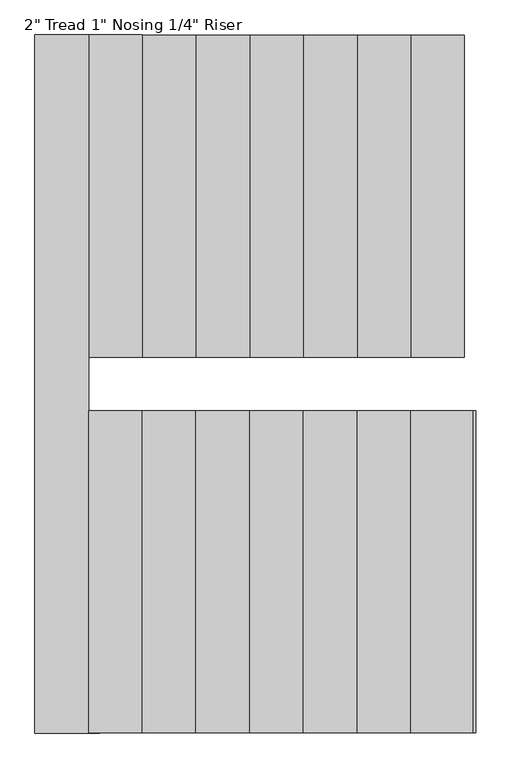
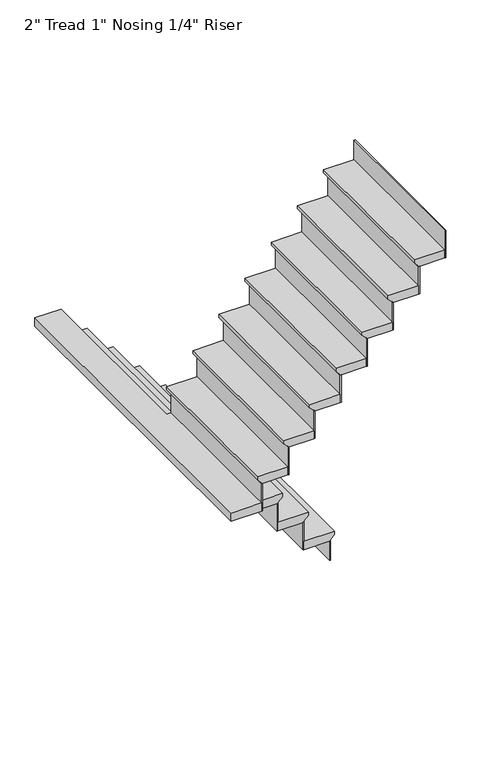
"""IFC4 building model written with IfcOpenShell, lengths in millimetres: stair flight geometry."""

from ifc_helpers import new_model, si_unit, origin, place, context, project, spatial, faceted_brep, source, transform, mapped, element, save


def stair_flight_41b76c56(model_context):
    return source(origin(), model_context, "Body", "Brep", [
        faceted_brep([(3632.2, 10909.3, 150.2833333), (3632.2, 10909.3, 169.3333333), (3632.2, 9994.9, 169.3333333), (3632.2, 9994.9, 150.2833333), (3606.8, 10909.3, 124.8833333), (3606.8, 9994.9, 124.8833333), (3454.4, 10909.3, 169.3333333), (3454.4, 9994.9, 169.3333333), (3606.8, 9994.9, 118.5333333), (3454.4, 9994.9, 118.5333333), (3454.4, 10909.3, 118.5333333), (3606.8, 10909.3, 118.5333333)], [[[0, 1, 2, 3]], [[4, 0, 3, 5]], [[2, 1, 6, 7]], [[8, 9, 10, 11]], [[2, 7, 9, 8, 5, 3]], [[8, 11, 4, 5]], [[6, 1, 0, 4, 11, 10]], [[7, 6, 10, 9]]]),
        faceted_brep([(3606.8, 10909.3, 118.5333333), (3606.8, 10909.3, 0.0), (3600.45, 10909.3, 0.0), (3600.45, 10909.3, 118.5333333), (3606.8, 9994.9, 118.5333333), (3600.45, 9994.9, 118.5333333), (3600.45, 9994.9, 0.0), (3606.8, 9994.9, 0.0)], [[[0, 1, 2, 3]], [[4, 5, 6, 7]], [[1, 0, 4, 7]], [[2, 1, 7, 6]], [[3, 2, 6, 5]], [[0, 3, 5, 4]]]),
        faceted_brep([(3454.4, 10909.3, 287.8666667), (3454.4, 10909.3, 118.5333333), (3448.05, 10909.3, 118.5333333), (3448.05, 10909.3, 287.8666667), (3454.4, 9994.9, 287.8666667), (3448.05, 9994.9, 287.8666667), (3448.05, 9994.9, 118.5333333), (3454.4, 9994.9, 118.5333333)], [[[0, 1, 2, 3]], [[4, 5, 6, 7]], [[1, 0, 4, 7]], [[2, 1, 7, 6]], [[3, 2, 6, 5]], [[0, 3, 5, 4]]]),
        faceted_brep([(3479.8, 9994.9, 338.6666667), (3479.8, 10909.3, 338.6666667), (3302.0, 10909.3, 338.6666667), (3302.0, 9994.9, 338.6666667), (3454.4, 9994.9, 287.8666667), (3302.0, 9994.9, 287.8666667), (3302.0, 10909.3, 287.8666667), (3454.4, 10909.3, 287.8666667), (3454.4, 9994.9, 294.2166667), (3479.8, 9994.9, 319.6166667), (3454.4, 10909.3, 294.2166667), (3479.8, 10909.3, 319.6166667)], [[[0, 1, 2, 3]], [[4, 5, 6, 7]], [[0, 3, 5, 4, 8, 9]], [[4, 7, 10, 8]], [[2, 1, 11, 10, 7, 6]], [[3, 2, 6, 5]], [[11, 1, 0, 9]], [[10, 11, 9, 8]]]),
        faceted_brep([(3302.0, 10909.3, 457.2), (3302.0, 10909.3, 287.8666667), (3295.65, 10909.3, 287.8666667), (3295.65, 10909.3, 457.2), (3302.0, 9994.9, 457.2), (3295.65, 9994.9, 457.2), (3295.65, 9994.9, 287.8666667), (3302.0, 9994.9, 287.8666667)], [[[0, 1, 2, 3]], [[4, 5, 6, 7]], [[1, 0, 4, 7]], [[2, 1, 7, 6]], [[3, 2, 6, 5]], [[0, 3, 5, 4]]]),
        faceted_brep([(3327.4, 9994.9, 508.0), (3327.4, 10909.3, 508.0), (3149.6, 10909.3, 508.0), (3149.6, 9994.9, 508.0), (3302.0, 9994.9, 457.2), (3149.6, 9994.9, 457.2), (3149.6, 10909.3, 457.2), (3302.0, 10909.3, 457.2), (3302.0, 9994.9, 463.55), (3327.4, 9994.9, 488.95), (3302.0, 10909.3, 463.55), (3327.4, 10909.3, 488.95)], [[[0, 1, 2, 3]], [[4, 5, 6, 7]], [[0, 3, 5, 4, 8, 9]], [[4, 7, 10, 8]], [[2, 1, 11, 10, 7, 6]], [[3, 2, 6, 5]], [[11, 1, 0, 9]], [[10, 11, 9, 8]]]),
        faceted_brep([(3149.6, 10909.3, 626.5333333), (3149.6, 10909.3, 457.2), (3143.25, 10909.3, 457.2), (3143.25, 10909.3, 626.5333333), (3149.6, 9994.9, 626.5333333), (3143.25, 9994.9, 626.5333333), (3143.25, 9994.9, 457.2), (3149.6, 9994.9, 457.2)], [[[0, 1, 2, 3]], [[4, 5, 6, 7]], [[1, 0, 4, 7]], [[2, 1, 7, 6]], [[3, 2, 6, 5]], [[0, 3, 5, 4]]]),
        faceted_brep([(3175.0, 9994.9, 677.3333333), (3175.0, 10909.3, 677.3333333), (2997.2, 10909.3, 677.3333333), (2997.2, 9994.9, 677.3333333), (3149.6, 9994.9, 626.5333333), (2997.2, 9994.9, 626.5333333), (2997.2, 10909.3, 626.5333333), (3149.6, 10909.3, 626.5333333), (3149.6, 9994.9, 632.8833333), (3175.0, 9994.9, 658.2833333), (3149.6, 10909.3, 632.8833333), (3175.0, 10909.3, 658.2833333)], [[[0, 1, 2, 3]], [[4, 5, 6, 7]], [[0, 3, 5, 4, 8, 9]], [[4, 7, 10, 8]], [[2, 1, 11, 10, 7, 6]], [[3, 2, 6, 5]], [[11, 1, 0, 9]], [[10, 11, 9, 8]]]),
        faceted_brep([(2997.2, 10909.3, 795.8666667), (2997.2, 10909.3, 626.5333333), (2990.85, 10909.3, 626.5333333), (2990.85, 10909.3, 795.8666667), (2997.2, 9994.9, 795.8666667), (2990.85, 9994.9, 795.8666667), (2990.85, 9994.9, 626.5333333), (2997.2, 9994.9, 626.5333333)], [[[0, 1, 2, 3]], [[4, 5, 6, 7]], [[1, 0, 4, 7]], [[2, 1, 7, 6]], [[3, 2, 6, 5]], [[0, 3, 5, 4]]]),
        faceted_brep([(3022.6, 9994.9, 846.6666667), (3022.6, 10909.3, 846.6666667), (2844.8, 10909.3, 846.6666667), (2844.8, 9994.9, 846.6666667), (2997.2, 9994.9, 795.8666667), (2844.8, 9994.9, 795.8666667), (2844.8, 10909.3, 795.8666667), (2997.2, 10909.3, 795.8666667), (2997.2, 9994.9, 802.2166667), (3022.6, 9994.9, 827.6166667), (2997.2, 10909.3, 802.2166667), (3022.6, 10909.3, 827.6166667)], [[[0, 1, 2, 3]], [[4, 5, 6, 7]], [[0, 3, 5, 4, 8, 9]], [[4, 7, 10, 8]], [[2, 1, 11, 10, 7, 6]], [[3, 2, 6, 5]], [[11, 1, 0, 9]], [[10, 11, 9, 8]]]),
        faceted_brep([(2844.8, 10909.3, 965.2), (2844.8, 10909.3, 795.8666667), (2838.45, 10909.3, 795.8666667), (2838.45, 10909.3, 965.2), (2844.8, 9994.9, 965.2), (2838.45, 9994.9, 965.2), (2838.45, 9994.9, 795.8666667), (2844.8, 9994.9, 795.8666667)], [[[0, 1, 2, 3]], [[4, 5, 6, 7]], [[1, 0, 4, 7]], [[2, 1, 7, 6]], [[3, 2, 6, 5]], [[0, 3, 5, 4]]]),
        faceted_brep([(2870.2, 9994.9, 1016.0), (2870.2, 10909.3, 1016.0), (2692.4, 10909.3, 1016.0), (2692.4, 9994.9, 1016.0), (2844.8, 9994.9, 965.2), (2692.4, 9994.9, 965.2), (2692.4, 10909.3, 965.2), (2844.8, 10909.3, 965.2), (2844.8, 9994.9, 971.55), (2870.2, 9994.9, 996.95), (2844.8, 10909.3, 971.55), (2870.2, 10909.3, 996.95)], [[[0, 1, 2, 3]], [[4, 5, 6, 7]], [[0, 3, 5, 4, 8, 9]], [[4, 7, 10, 8]], [[2, 1, 11, 10, 7, 6]], [[3, 2, 6, 5]], [[11, 1, 0, 9]], [[10, 11, 9, 8]]]),
        faceted_brep([(2692.4, 10909.3, 1134.5333333), (2692.4, 10909.3, 965.2), (2686.05, 10909.3, 965.2), (2686.05, 10909.3, 1134.5333333), (2692.4, 9994.9, 1134.5333333), (2686.05, 9994.9, 1134.5333333), (2686.05, 9994.9, 965.2), (2692.4, 9994.9, 965.2)], [[[0, 1, 2, 3]], [[4, 5, 6, 7]], [[1, 0, 4, 7]], [[2, 1, 7, 6]], [[3, 2, 6, 5]], [[0, 3, 5, 4]]]),
        faceted_brep([(2717.8, 9994.9, 1185.3333333), (2717.8, 10909.3, 1185.3333333), (2540.0, 10909.3, 1185.3333333), (2540.0, 9994.9, 1185.3333333), (2692.4, 9994.9, 1134.5333333), (2540.0, 9994.9, 1134.5333333), (2540.0, 10909.3, 1134.5333333), (2692.4, 10909.3, 1134.5333333), (2692.4, 9994.9, 1140.8833333), (2717.8, 9994.9, 1166.2833333), (2692.4, 10909.3, 1140.8833333), (2717.8, 10909.3, 1166.2833333)], [[[0, 1, 2, 3]], [[4, 5, 6, 7]], [[0, 3, 5, 4, 8, 9]], [[4, 7, 10, 8]], [[2, 1, 11, 10, 7, 6]], [[3, 2, 6, 5]], [[11, 1, 0, 9]], [[10, 11, 9, 8]]]),
        faceted_brep([(2540.0, 10909.3, 1303.8666667), (2540.0, 10909.3, 1134.5333333), (2533.65, 10909.3, 1134.5333333), (2533.65, 10909.3, 1303.8666667), (2540.0, 9994.9, 1303.8666667), (2533.65, 9994.9, 1303.8666667), (2533.65, 9994.9, 1134.5333333), (2540.0, 9994.9, 1134.5333333)], [[[0, 1, 2, 3]], [[4, 5, 6, 7]], [[1, 0, 4, 7]], [[2, 1, 7, 6]], [[3, 2, 6, 5]], [[0, 3, 5, 4]]]),
        faceted_brep([(2590.8, 9842.5, 1354.6666667), (2565.4, 9842.5, 1354.6666667), (2565.4, 10909.3, 1354.6666667), (2413.0, 10909.3, 1354.6666667), (2413.0, 8928.1, 1354.6666667), (2590.8, 8928.1, 1354.6666667), (2565.4, 9842.5, 1303.8666667), (2590.8, 9842.5, 1303.8666667), (2590.8, 8928.1, 1303.8666667), (2413.0, 8928.1, 1303.8666667), (2413.0, 10909.3, 1303.8666667), (2540.0, 10909.3, 1303.8666667), (2540.0, 9994.9, 1303.8666667), (2565.4, 9994.9, 1303.8666667), (2565.4, 9994.9, 1335.6166667), (2565.4, 10909.3, 1335.6166667), (2540.0, 9994.9, 1310.2166667), (2540.0, 10909.3, 1310.2166667)], [[[0, 1, 2, 3, 4, 5]], [[6, 7, 8, 9, 10, 11, 12, 13]], [[1, 0, 7, 6]], [[2, 1, 6, 13, 14, 15]], [[13, 12, 16, 14]], [[12, 11, 17, 16]], [[3, 2, 15, 17, 11, 10]], [[4, 3, 10, 9]], [[5, 4, 9, 8]], [[0, 5, 8, 7]], [[17, 15, 14, 16]]]),
        faceted_brep([(2590.8, 8928.1, 1473.2), (2590.8, 8928.1, 1303.8666667), (2597.15, 8928.1, 1303.8666667), (2597.15, 8928.1, 1473.2), (2590.8, 9842.5, 1473.2), (2597.15, 9842.5, 1473.2), (2597.15, 9842.5, 1303.8666667), (2590.8, 9842.5, 1303.8666667)], [[[0, 1, 2, 3]], [[4, 5, 6, 7]], [[1, 0, 4, 7]], [[2, 1, 7, 6]], [[3, 2, 6, 5]], [[0, 3, 5, 4]]]),
        faceted_brep([(2565.4, 9842.5, 1524.0), (2565.4, 8928.1, 1524.0), (2743.2, 8928.1, 1524.0), (2743.2, 9842.5, 1524.0), (2590.8, 9842.5, 1473.2), (2743.2, 9842.5, 1473.2), (2743.2, 8928.1, 1473.2), (2590.8, 8928.1, 1473.2), (2590.8, 9842.5, 1479.55), (2565.4, 9842.5, 1504.95), (2590.8, 8928.1, 1479.55), (2565.4, 8928.1, 1504.95)], [[[0, 1, 2, 3]], [[4, 5, 6, 7]], [[0, 3, 5, 4, 8, 9]], [[4, 7, 10, 8]], [[2, 1, 11, 10, 7, 6]], [[3, 2, 6, 5]], [[11, 1, 0, 9]], [[10, 11, 9, 8]]]),
        faceted_brep([(2743.2, 8928.1, 1642.5333333), (2743.2, 8928.1, 1473.2), (2749.55, 8928.1, 1473.2), (2749.55, 8928.1, 1642.5333333), (2743.2, 9842.5, 1642.5333333), (2749.55, 9842.5, 1642.5333333), (2749.55, 9842.5, 1473.2), (2743.2, 9842.5, 1473.2)], [[[0, 1, 2, 3]], [[4, 5, 6, 7]], [[1, 0, 4, 7]], [[2, 1, 7, 6]], [[3, 2, 6, 5]], [[0, 3, 5, 4]]]),
        faceted_brep([(2717.8, 9842.5, 1693.3333333), (2717.8, 8928.1, 1693.3333333), (2895.6, 8928.1, 1693.3333333), (2895.6, 9842.5, 1693.3333333), (2743.2, 9842.5, 1642.5333333), (2895.6, 9842.5, 1642.5333333), (2895.6, 8928.1, 1642.5333333), (2743.2, 8928.1, 1642.5333333), (2743.2, 9842.5, 1648.8833333), (2717.8, 9842.5, 1674.2833333), (2743.2, 8928.1, 1648.8833333), (2717.8, 8928.1, 1674.2833333)], [[[0, 1, 2, 3]], [[4, 5, 6, 7]], [[0, 3, 5, 4, 8, 9]], [[4, 7, 10, 8]], [[2, 1, 11, 10, 7, 6]], [[3, 2, 6, 5]], [[11, 1, 0, 9]], [[10, 11, 9, 8]]]),
        faceted_brep([(2895.6, 8928.1, 1811.8666667), (2895.6, 8928.1, 1642.5333333), (2901.95, 8928.1, 1642.5333333), (2901.95, 8928.1, 1811.8666667), (2895.6, 9842.5, 1811.8666667), (2901.95, 9842.5, 1811.8666667), (2901.95, 9842.5, 1642.5333333), (2895.6, 9842.5, 1642.5333333)], [[[0, 1, 2, 3]], [[4, 5, 6, 7]], [[1, 0, 4, 7]], [[2, 1, 7, 6]], [[3, 2, 6, 5]], [[0, 3, 5, 4]]]),
        faceted_brep([(2870.2, 9842.5, 1862.6666667), (2870.2, 8928.1, 1862.6666667), (3048.0, 8928.1, 1862.6666667), (3048.0, 9842.5, 1862.6666667), (2895.6, 9842.5, 1811.8666667), (3048.0, 9842.5, 1811.8666667), (3048.0, 8928.1, 1811.8666667), (2895.6, 8928.1, 1811.8666667), (2895.6, 9842.5, 1818.2166667), (2870.2, 9842.5, 1843.6166667), (2895.6, 8928.1, 1818.2166667), (2870.2, 8928.1, 1843.6166667)], [[[0, 1, 2, 3]], [[4, 5, 6, 7]], [[0, 3, 5, 4, 8, 9]], [[4, 7, 10, 8]], [[2, 1, 11, 10, 7, 6]], [[3, 2, 6, 5]], [[11, 1, 0, 9]], [[10, 11, 9, 8]]]),
        faceted_brep([(3048.0, 8928.1, 1981.2), (3048.0, 8928.1, 1811.8666667), (3054.35, 8928.1, 1811.8666667), (3054.35, 8928.1, 1981.2), (3048.0, 9842.5, 1981.2), (3054.35, 9842.5, 1981.2), (3054.35, 9842.5, 1811.8666667), (3048.0, 9842.5, 1811.8666667)], [[[0, 1, 2, 3]], [[4, 5, 6, 7]], [[1, 0, 4, 7]], [[2, 1, 7, 6]], [[3, 2, 6, 5]], [[0, 3, 5, 4]]]),
        faceted_brep([(3022.6, 9842.5, 2032.0), (3022.6, 8928.1, 2032.0), (3200.4, 8928.1, 2032.0), (3200.4, 9842.5, 2032.0), (3048.0, 9842.5, 1981.2), (3200.4, 9842.5, 1981.2), (3200.4, 8928.1, 1981.2), (3048.0, 8928.1, 1981.2), (3048.0, 9842.5, 1987.55), (3022.6, 9842.5, 2012.95), (3048.0, 8928.1, 1987.55), (3022.6, 8928.1, 2012.95)], [[[0, 1, 2, 3]], [[4, 5, 6, 7]], [[0, 3, 5, 4, 8, 9]], [[4, 7, 10, 8]], [[2, 1, 11, 10, 7, 6]], [[3, 2, 6, 5]], [[11, 1, 0, 9]], [[10, 11, 9, 8]]]),
        faceted_brep([(3200.4, 8928.1, 2150.5333333), (3200.4, 8928.1, 1981.2), (3206.75, 8928.1, 1981.2), (3206.75, 8928.1, 2150.5333333), (3200.4, 9842.5, 2150.5333333), (3206.75, 9842.5, 2150.5333333), (3206.75, 9842.5, 1981.2), (3200.4, 9842.5, 1981.2)], [[[0, 1, 2, 3]], [[4, 5, 6, 7]], [[1, 0, 4, 7]], [[2, 1, 7, 6]], [[3, 2, 6, 5]], [[0, 3, 5, 4]]]),
        faceted_brep([(3175.0, 9842.5, 2201.3333333), (3175.0, 8928.1, 2201.3333333), (3352.8, 8928.1, 2201.3333333), (3352.8, 9842.5, 2201.3333333), (3200.4, 9842.5, 2150.5333333), (3352.8, 9842.5, 2150.5333333), (3352.8, 8928.1, 2150.5333333), (3200.4, 8928.1, 2150.5333333), (3200.4, 9842.5, 2156.8833333), (3175.0, 9842.5, 2182.2833333), (3200.4, 8928.1, 2156.8833333), (3175.0, 8928.1, 2182.2833333)], [[[0, 1, 2, 3]], [[4, 5, 6, 7]], [[0, 3, 5, 4, 8, 9]], [[4, 7, 10, 8]], [[2, 1, 11, 10, 7, 6]], [[3, 2, 6, 5]], [[11, 1, 0, 9]], [[10, 11, 9, 8]]]),
        faceted_brep([(3352.8, 8928.1, 2319.8666667), (3352.8, 8928.1, 2150.5333333), (3359.15, 8928.1, 2150.5333333), (3359.15, 8928.1, 2319.8666667), (3352.8, 9842.5, 2319.8666667), (3359.15, 9842.5, 2319.8666667), (3359.15, 9842.5, 2150.5333333), (3352.8, 9842.5, 2150.5333333)], [[[0, 1, 2, 3]], [[4, 5, 6, 7]], [[1, 0, 4, 7]], [[2, 1, 7, 6]], [[3, 2, 6, 5]], [[0, 3, 5, 4]]]),
        faceted_brep([(3327.4, 9842.5, 2370.6666667), (3327.4, 8928.1, 2370.6666667), (3505.2, 8928.1, 2370.6666667), (3505.2, 9842.5, 2370.6666667), (3352.8, 9842.5, 2319.8666667), (3505.2, 9842.5, 2319.8666667), (3505.2, 8928.1, 2319.8666667), (3352.8, 8928.1, 2319.8666667), (3352.8, 9842.5, 2326.2166667), (3327.4, 9842.5, 2351.6166667), (3352.8, 8928.1, 2326.2166667), (3327.4, 8928.1, 2351.6166667)], [[[0, 1, 2, 3]], [[4, 5, 6, 7]], [[0, 3, 5, 4, 8, 9]], [[4, 7, 10, 8]], [[2, 1, 11, 10, 7, 6]], [[3, 2, 6, 5]], [[11, 1, 0, 9]], [[10, 11, 9, 8]]]),
        faceted_brep([(3505.2, 8928.1, 2489.2), (3505.2, 8928.1, 2319.8666667), (3511.55, 8928.1, 2319.8666667), (3511.55, 8928.1, 2489.2), (3505.2, 9842.5, 2489.2), (3511.55, 9842.5, 2489.2), (3511.55, 9842.5, 2319.8666667), (3505.2, 9842.5, 2319.8666667)], [[[0, 1, 2, 3]], [[4, 5, 6, 7]], [[1, 0, 4, 7]], [[2, 1, 7, 6]], [[3, 2, 6, 5]], [[0, 3, 5, 4]]]),
        faceted_brep([(3657.6, 8928.1, 2658.5333333), (3657.6, 8928.1, 2489.2), (3663.95, 8928.1, 2489.2), (3663.95, 8928.1, 2658.5333333), (3657.6, 9842.5, 2658.5333333), (3663.95, 9842.5, 2658.5333333), (3663.95, 9842.5, 2489.2), (3657.6, 9842.5, 2489.2)], [[[0, 1, 2, 3]], [[4, 5, 6, 7]], [[1, 0, 4, 7]], [[2, 1, 7, 6]], [[3, 2, 6, 5]], [[0, 3, 5, 4]]]),
        faceted_brep([(3479.8, 9842.5, 2540.0), (3479.8, 8928.1, 2540.0), (3657.6, 8928.1, 2540.0), (3657.6, 9842.5, 2540.0), (3505.2, 9842.5, 2489.2), (3657.6, 9842.5, 2489.2), (3657.6, 8928.1, 2489.2), (3505.2, 8928.1, 2489.2), (3505.2, 9842.5, 2495.55), (3479.8, 9842.5, 2520.95), (3505.2, 8928.1, 2495.55), (3479.8, 8928.1, 2520.95)], [[[0, 1, 2, 3]], [[4, 5, 6, 7]], [[0, 3, 5, 4, 8, 9]], [[4, 7, 10, 8]], [[2, 1, 11, 10, 7, 6]], [[3, 2, 6, 5]], [[11, 1, 0, 9]], [[10, 11, 9, 8]]]),
    ])


if __name__ == "__main__":
    model = new_model("IFC4")
    model_context = context("Model", 3, world=origin())
    ifc_project = project(units=[si_unit("LENGTHUNIT", "METRE", prefix="MILLI")], contexts=[model_context])
    site = spatial("IfcSite", under=ifc_project)
    building = spatial("IfcBuilding", under=site)
    placement = place(None, origin())
    stair_flight_shape = stair_flight_41b76c56(model_context)
    element("IfcStairFlight", 1, ObjectType="2\" Tread 1\" Nosing 1/4\" Riser", at=placement, inside=building, context=model_context, shape_type="MappedRepresentation", body=[
        mapped(stair_flight_shape, transform((0.0, 0.0, 0.0), x_axis=(1.0, 0.0, 0.0), y_axis=(0.0, 1.0, 0.0), z_axis=(0.0, 0.0, 1.0))),
    ])
    save(model, "model.ifc")
